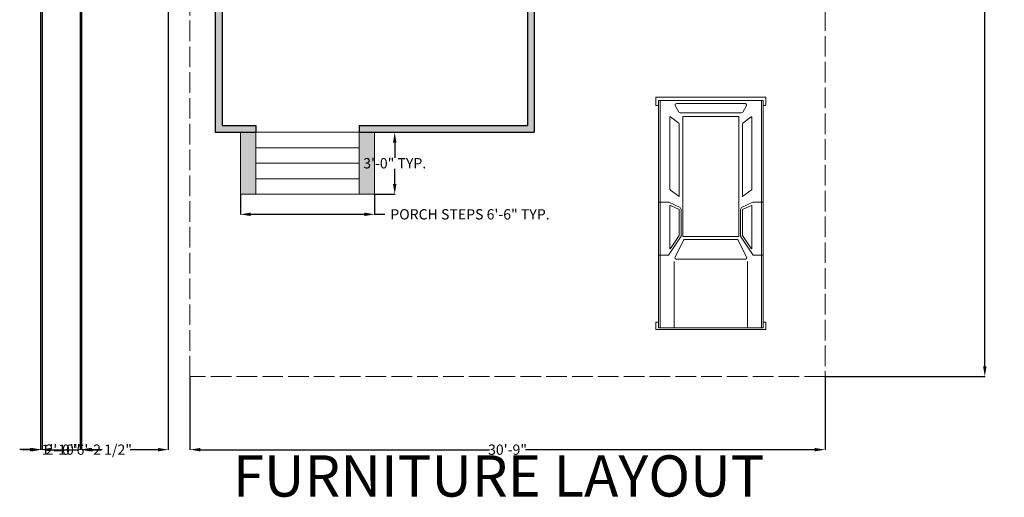
# Model space of a CAD drawing. Units: inches. Extents: x 1966 to 4198, y 2607 to 3884.
# Tile 4 of 8: x 2877 to 3450, y 3133 to 3411. Entities that reach past the tile are written whole.
import ezdxf

# ---------------------------------------------------------------- set-up
doc = ezdxf.new("R2010")
doc.units = ezdxf.units.IN
doc.header["$MEASUREMENT"] = 0
doc.linetypes.add('ACAD_ISO02W100', pattern=[15, 12, -3])
for name, color, linetype, lineweight in [('A-ANNO-TEXT', 4, 'Continuous', 25), ('A-FLOR', 7, 'Continuous', 25), ('A-FLOR-PATT', 9, 'Continuous', 13), ('A-FLOR-STRS', 7, 'Continuous', 18), ('A-WALL-PATT', 252, 'Continuous', 13), ('C-PRKG', 10, 'ACAD_ISO02W100', 18), ('C-PRKG-VEHI', 163, 'Continuous', 18), ('dimension', 90, 'Continuous', 18)]:
    doc.layers.add(name, color=color, linetype=linetype, lineweight=lineweight)
doc.styles.get("Standard").update_dxf_attribs({"font": 'arial.ttf'})
doc.dimstyles.get("Standard").update_dxf_attribs({"dimtxt": 6, "dimasz": 6, "dimexe": 0.18, "dimexo": 0.0625, "dimgap": 0.09, "dimtad": 0, "dimtih": 1, "dimtoh": 1, "dimdec": 1, "dimzin": 0, "dimdsep": 46, "dimlunit": 3, "dimtxsty": 'Standard', "dimcen": 0.09, "dimadec": 0, "dimazin": 0, "dimtfac": 1, "dimtdec": 1, "dimtofl": 0, "dimtmove": 0, "dimatfit": 3, "dimfxl": 1, "dimtolj": 1, "dimtzin": 0, "dimarcsym": 0})

# ---------------------------------------------------------------- blocks, each defined once
blk = doc.blocks.new('*U12')
for p, q in [((1.28, 38.87), (175.66, 38.87)), ((1.28, 28.15), (52.13, 28.15)), ((1.28, -28.15), (52.13, -28.15)), ((1.28, -38.87), (175.66, -38.87))]:
    blk.add_line(p, q)
for points in [[(5.57, 40.01), (5.57, 42.18), (0, 42.18), (0, -42.18), (5.57, -42.18), (5.57, -40.01), (1.28, -40.01), (1.28, 40.01)], [(1.28, 40.01), (175.66, 40.01), (175.66, -40.01), (1.28, -40.01)], [(171.74, 40.01), (175.66, 40.01), (175.66, -40.01), (171.74, -40.01), (171.74, -42.18), (178.14, -42.18), (178.14, 42.18), (171.74, 42.18)], [(71.47, 21.48), (163.42, 21.48), (163.42, -21.48), (71.47, -21.48)]]:
    blk.add_lwpolyline(points, close=True)
for points in [[(57.15, 40.01), (57.15, 32.39), (71.72, 22.83, 0.086577), (72.56, 22.68), (91.59, 22.68, 0.227875), (93.54, 23.62), (97.72, 32.11), (97.72, 40.01)], [(57.15, -40.01), (57.15, -32.39), (71.72, -22.83, -0.086577), (72.56, -22.68), (91.59, -22.68, -0.227875), (93.54, -23.62), (97.72, -32.11), (97.72, -40.01)]]:
    blk.add_lwpolyline(points, format="xyb")
for points in [[(62.08, 30.95), (72.14, 24.35, 0.146139), (72.69, 24.18), (91.42, 24.18, 0.29766), (92.33, 24.78), (95.09, 31.05, 0.541236), (94.86, 31.41), (62.21, 31.41, 0.744989)], [(102.19, 24.58), (106.97, 31, -0.236929), (107.78, 31.41), (162.91, 31.41, -0.621576), (163.11, 31), (158.19, 24.58, -0.233368), (157.39, 24.18), (102.39, 24.18, -0.616908)], [(55.49, 27.42), (68.59, 20.89, -0.284287), (69.14, 19.99), (69.14, -19.99, -0.284287), (68.59, -20.89), (55.49, -27.42, -0.557284), (54.05, -26.53), (54.05, 26.53, -0.557284)], [(171.88, 27.31), (166.83, 24.47, 0.271143), (166.32, 23.6), (166.32, -23.6, 0.271143), (166.83, -24.47), (171.88, -27.31, 0.573387), (173.37, -26.44), (173.37, 26.44, 0.573387)], [(62.08, -30.95), (72.14, -24.35, -0.146139), (72.69, -24.18), (91.42, -24.18, -0.29766), (92.33, -24.78), (95.09, -31.05, -0.541236), (94.86, -31.41), (62.21, -31.41, -0.744989)], [(102.19, -24.58), (106.97, -31, 0.236929), (107.78, -31.41), (162.91, -31.41, 0.621576), (163.11, -31), (158.19, -24.58, 0.233368), (157.39, -24.18), (102.39, -24.18, 0.616908)]]:
    blk.add_lwpolyline(points, format="xyb", close=True)
blk = doc.blocks.new('PORCH-ENTRY-STEPS')
for p, q in [((0, 36), (0, 0)), ((9, 36), (9, 0)), ((9, 36), (69, 36)), ((69, 0), (69, 36)), ((78, 0), (78, 36)), ((9, 27), (69, 27)), ((9, 18), (69, 18)), ((9, 9), (69, 9)), ((9, 0), (0, 0)), ((9, 0), (69, 0)), ((69, 0), (78, 0))]:
    blk.add_line(p, q)
blk = doc.blocks.new('PORCH-PARAPET-PLAN')
for p, q in [((0, 86), (0, 0)), ((4, 86), (4, 4)), ((181.42, 86), (181.42, 4)), ((185.42, 86), (185.42, 0)), ((0, 0), (23.64, 0)), ((4, 4), (23.64, 4)), ((23.64, 4), (23.64, 0)), ((83.64, 4), (83.64, 0)), ((83.64, 4), (181.42, 4)), ((83.64, 0), (185.42, 0))]:
    blk.add_line(p, q)
blk = doc.blocks.new('*D57')
at = {"layer": 'Defpoints', "color": 0, "transparency": 16777216}
for p in [(3005.67, 3309.5), (3083.67, 3309.5), (3083.67, 3297.8)]:
    blk.add_point(p, dxfattribs=at)
at = {"layer": 'dimension', "color": 0, "lineweight": -2, "transparency": 16777216}
for p, q in [((3005.67, 3309.44), (3005.67, 3297.62)), ((3083.67, 3309.44), (3083.67, 3297.62)), ((3011.67, 3297.8), (3077.67, 3297.8)), ((3083.67, 3297.8), (3089.67, 3297.8))]:
    blk.add_line(p, q, dxfattribs=at)
at = {"layer": 'dimension', "color": 0, "transparency": 16777216}
for points in [[(3011.67, 3298.8), (3011.67, 3296.8), (3005.67, 3297.8)], [(3077.67, 3298.8), (3077.67, 3296.8), (3083.67, 3297.8)]]:
    blk.add_solid(points, dxfattribs=at)
at = {"layer": 'dimension', "color": 0, "transparency": 16777216, "insert": (3139.1, 3297.8), "char_height": 6, "attachment_point": 5}
blk.add_mtext('\\A1;PORCH STEPS 6\'-6" TYP.', dxfattribs=at)
blk = doc.blocks.new('*D58')
at = {"layer": 'Defpoints', "color": 0, "transparency": 16777216}
for p in [(3083.67, 3345.5), (3095.37, 3345.5), (3083.67, 3309.5)]:
    blk.add_point(p, dxfattribs=at)
at = {"layer": 'dimension', "color": 0, "lineweight": -2, "transparency": 16777216}
for p, q in [((3083.73, 3345.5), (3095.55, 3345.5)), ((3095.37, 3339.5), (3095.37, 3330.66)), ((3095.37, 3315.5), (3095.37, 3324.35)), ((3083.73, 3309.5), (3095.55, 3309.5))]:
    blk.add_line(p, q, dxfattribs=at)
at = {"layer": 'dimension', "color": 0, "transparency": 16777216}
for points in [[(3094.37, 3339.5), (3096.37, 3339.5), (3095.37, 3345.5)], [(3094.37, 3315.5), (3096.37, 3315.5), (3095.37, 3309.5)]]:
    blk.add_solid(points, dxfattribs=at)
at = {"layer": 'dimension', "color": 0, "transparency": 16777216, "insert": (3095.37, 3327.5), "char_height": 6, "attachment_point": 5}
blk.add_mtext('\\A1;3\'-0" TYP.', dxfattribs=at)
blk = doc.blocks.new('*D88')
at = {"layer": 'Defpoints', "color": 0, "transparency": 16777216}
for p in [(3058.44, 3836.5), (3345.44, 3203.44), (3438.28, 3203.44)]:
    blk.add_point(p, dxfattribs=at)
at = {"layer": 'dimension', "color": 0, "lineweight": -2, "transparency": 16777216}
for p, q in [((3058.5, 3836.5), (3438.46, 3836.5)), ((3438.28, 3830.5), (3438.28, 3523.13)), ((3438.28, 3209.44), (3438.28, 3516.82)), ((3345.5, 3203.44), (3438.46, 3203.44))]:
    blk.add_line(p, q, dxfattribs=at)
at = {"layer": 'dimension', "color": 0, "transparency": 16777216}
for points in [[(3437.28, 3830.5), (3439.28, 3830.5), (3438.28, 3836.5)], [(3437.28, 3209.44), (3439.28, 3209.44), (3438.28, 3203.44)]]:
    blk.add_solid(points, dxfattribs=at)
at = {"layer": 'dimension', "color": 0, "transparency": 16777216, "insert": (3438.28, 3519.97), "char_height": 6, "attachment_point": 5}
blk.add_mtext('\\A1;52\'-9"', dxfattribs=at)
blk = doc.blocks.new('*D89')
at = {"layer": 'Defpoints', "color": 0, "transparency": 16777216}
for p in [(2976.4, 3203.44), (3345.44, 3203.44), (3345.44, 3160.93)]:
    blk.add_point(p, dxfattribs=at)
at = {"layer": 'dimension', "color": 0, "lineweight": -2, "transparency": 16777216}
for p, q in [((2976.4, 3203.38), (2976.4, 3160.75)), ((3345.44, 3203.38), (3345.44, 3160.75)), ((2982.4, 3160.93), (3150.53, 3160.93)), ((3339.44, 3160.93), (3171.31, 3160.93))]:
    blk.add_line(p, q, dxfattribs=at)
at = {"layer": 'dimension', "color": 0, "transparency": 16777216}
for points in [[(2982.4, 3161.93), (2982.4, 3159.93), (2976.4, 3160.93)], [(3339.44, 3161.93), (3339.44, 3159.93), (3345.44, 3160.93)]]:
    blk.add_solid(points, dxfattribs=at)
at = {"layer": 'dimension', "color": 0, "transparency": 16777216, "insert": (3160.92, 3160.93), "char_height": 6, "attachment_point": 5}
blk.add_mtext('\\A1;30\'-9"', dxfattribs=at)
blk = doc.blocks.new('*D90')
at = {"layer": 'Defpoints', "color": 0, "transparency": 16777216}
for p in [(2889.440566, 3668.990639), (2913.440566, 3668.990639), (2913.440566, 3160.931053)]:
    blk.add_point(p, dxfattribs=at)
at = {"layer": 'dimension', "color": 0, "lineweight": -2, "transparency": 16777216}
for p, q in [((2889.440566, 3668.928139), (2889.440566, 3160.751053)), ((2913.440566, 3668.928139), (2913.440566, 3160.751053)), ((2883.440566, 3160.931053), (2877.440566, 3160.931053)), ((2919.440566, 3160.931053), (2925.440566, 3160.931053))]:
    blk.add_line(p, q, dxfattribs=at)
at = {"layer": 'dimension', "color": 0, "transparency": 16777216}
for points in [[(2883.440566, 3161.931053), (2883.440566, 3159.931053), (2889.440566, 3160.931053)], [(2919.440566, 3161.931053), (2919.440566, 3159.931053), (2913.440566, 3160.931053)]]:
    blk.add_solid(points, dxfattribs=at)
at = {"layer": 'dimension', "color": 0, "transparency": 16777216, "insert": (2901.440566, 3160.931053), "char_height": 6, "attachment_point": 5}
blk.add_mtext('\\A1;2\'-0"', dxfattribs=at)
blk = doc.blocks.new('*D92')
at = {"layer": 'Defpoints', "color": 0, "transparency": 16777216}
for p in [(2889.44, 3623.5), (2963.74, 3623.5), (2963.74, 3160.93)]:
    blk.add_point(p, dxfattribs=at)
at = {"layer": 'dimension', "color": 0, "lineweight": -2, "transparency": 16777216}
for p, q in [((2889.44, 3623.44), (2889.44, 3160.75)), ((2963.74, 3623.44), (2963.74, 3160.75)), ((2895.44, 3160.93), (2911.52, 3160.93)), ((2957.74, 3160.93), (2941.66, 3160.93))]:
    blk.add_line(p, q, dxfattribs=at)
at = {"layer": 'dimension', "color": 0, "transparency": 16777216}
for points in [[(2895.44, 3161.93), (2895.44, 3159.93), (2889.44, 3160.93)], [(2957.74, 3161.93), (2957.74, 3159.93), (2963.74, 3160.93)]]:
    blk.add_solid(points, dxfattribs=at)
at = {"layer": 'dimension', "color": 0, "transparency": 16777216, "insert": (2926.59, 3160.93), "char_height": 6, "attachment_point": 5}
blk.add_mtext('\\A1;6\'-2 1/2"', dxfattribs=at)
blk = doc.blocks.new('*D97')
at = {"layer": 'Defpoints', "color": 0, "transparency": 16777216}
for p in [(2890.43, 3707.11), (2912.55, 3707.11), (2912.55, 3160.93)]:
    blk.add_point(p, dxfattribs=at)
at = {"layer": 'dimension', "color": 0, "lineweight": -2, "transparency": 16777216}
for p, q in [((2890.43, 3707.05), (2890.43, 3160.75)), ((2912.55, 3707.05), (2912.55, 3160.75)), ((2884.43, 3160.93), (2878.43, 3160.93)), ((2918.55, 3160.93), (2924.55, 3160.93))]:
    blk.add_line(p, q, dxfattribs=at)
at = {"layer": 'dimension', "color": 0, "transparency": 16777216}
for points in [[(2884.43, 3161.93), (2884.43, 3159.93), (2890.43, 3160.93)], [(2918.55, 3161.93), (2918.55, 3159.93), (2912.55, 3160.93)]]:
    blk.add_solid(points, dxfattribs=at)
at = {"layer": 'dimension', "color": 0, "transparency": 16777216, "insert": (2901.49, 3160.93), "char_height": 6, "attachment_point": 5}
blk.add_mtext('\\A1;1\'-10"', dxfattribs=at)

msp = doc.modelspace()

# ---------------------------------------------------------------- hatches: boundary and pattern name
at = {"layer": 'A-FLOR-PATT'}
h = msp.add_hatch(color=256, dxfattribs=at)
h.dxf.hatch_style = 1
h.paths.add_polyline_path([(3014.67, 3345.5), (3005.67, 3345.5), (3005.67, 3309.5), (3014.67, 3309.5)])
h.paths.add_polyline_path([(3083.67, 3345.5), (3074.67, 3345.5), (3074.67, 3309.5), (3083.67, 3309.5)])
at = {"layer": 'A-WALL-PATT'}
h = msp.add_hatch(color=256, dxfattribs=at)
h.dxf.hatch_style = 1
h.paths.add_polyline_path([(3010.44, 3599.5), (2889.44, 3599.5), (2889.44, 3698.62), (2880.44, 3698.62), (2880.44, 3590.5), (2880.44, 3539.5), (2889.44, 3539.5), (2889.44, 3590.5), (3010.44, 3590.5)])
h.paths.add_polyline_path([(2889.44, 3491.5), (2880.44, 3491.5), (2880.44, 3431.5), (2924.93, 3431.5), (2924.93, 3440.5), (2889.44, 3440.5)])
h.paths.add_polyline_path([(3008.43, 3440.5), (2972.93, 3440.5), (2972.93, 3431.5), (3008.43, 3431.5)])
h.paths.add_polyline_path([(2995.02, 3431.5), (2991.02, 3431.5), (2991.02, 3345.5), (3014.67, 3345.5), (3014.67, 3349.5), (2995.02, 3349.5)])
h.paths.add_polyline_path([(3232.44, 3440.5), (3176.44, 3440.5), (3176.44, 3587.5), (3183.92, 3587.5), (3183.92, 3591.41), (3183.92, 3596.5), (3167.44, 3596.5), (3167.44, 3440.5), (3092.44, 3440.5), (3092.44, 3590.5), (3083.44, 3590.5), (3083.44, 3440.5), (3056.43, 3440.5), (3056.43, 3438.68), (3056.43, 3431.5), (3092.44, 3431.5), (3232.44, 3431.5)])
h.paths.add_polyline_path([(3176.44, 3431.5), (3172.44, 3431.5), (3172.44, 3349.5), (3074.67, 3349.5), (3074.67, 3345.5), (3176.44, 3345.5)])
h.paths.add_polyline_path([(3345.44, 3490), (3336.44, 3490), (3336.44, 3440.5), (3280.44, 3440.5), (3280.44, 3431.5), (3345.44, 3431.5)])
h.paths.add_polyline_path([(3345.44, 3599.5), (3345.44, 3602.5), (3336.44, 3602.5), (3336.44, 3596.5), (3296.55, 3596.5), (3296.55, 3587.5), (3336.44, 3587.5), (3336.44, 3538), (3345.44, 3538)])
h.paths.add_polyline_path([(3264.44, 3632.5), (3336.44, 3632.5), (3336.44, 3626.5), (3345.44, 3626.5), (3345.44, 3692.5), (3336.44, 3692.5), (3336.44, 3641.5), (3219.92, 3641.5), (3219.92, 3632.5), (3258.44, 3632.5), (3258.44, 3596.5), (3219.95, 3596.5), (3219.95, 3591.41, -0.010779), (3219.92, 3589.86), (3219.92, 3587.5), (3268.55, 3587.5), (3268.55, 3591.7), (3268.55, 3596.5), (3264.44, 3596.5)])
h.paths.add_polyline_path([(3175.44, 3791.5), (3231.94, 3791.5), (3231.94, 3800.5), (3175.44, 3800.5), (3154.44, 3800.5), (3154.44, 3791.5), (3166.44, 3791.5), (3166.44, 3719.5), (3118.44, 3719.5), (3112.44, 3719.5), (3058.44, 3719.5), (3058.44, 3710.5), (3166.44, 3710.5), (3166.44, 3632.5), (3183.92, 3632.5), (3183.92, 3637.87), (3183.92, 3641.5), (3175.44, 3641.5)])
h.paths.add_polyline_path([(3345.44, 3800.5), (3279.94, 3800.5), (3279.94, 3791.5), (3336.44, 3791.5), (3336.44, 3740.5), (3345.44, 3740.5)])
h.paths.add_polyline_path([(3130.44, 3800.5), (3100.44, 3800.5), (3100.44, 3791.5), (3112.44, 3791.5), (3112.44, 3755.5), (3112.44, 3751.71), (3112.44, 3747.5), (3118.44, 3747.5), (3118.44, 3791.5), (3130.44, 3791.5)], flags=17)
h.paths.add_polyline_path([(3076.44, 3800.5), (3058.44, 3800.5), (3058.44, 3796.92), (3058.44, 3791.5), (3058.44, 3749.5), (3084.38, 3749.5), (3084.38, 3751.71, -0.016709), (3084.44, 3753.59), (3084.44, 3755.5), (3064.44, 3755.5), (3064.44, 3791.5), (3076.44, 3791.5)], flags=17)
h.paths.add_polyline_path([(3022.36, 3796.92, -0.017138), (3022.44, 3799.39), (3022.44, 3800.5), (3010.44, 3800.5), (2969.44, 3800.5), (2969.44, 3791.5), (3001.44, 3791.5), (3001.44, 3632.5), (3010.44, 3632.5), (3010.44, 3791.5), (3022.36, 3791.5)])
h.paths.add_polyline_path([(2921.44, 3800.5), (2880.44, 3800.5), (2880.44, 3746.62), (2889.44, 3746.62), (2889.44, 3791.5), (2921.44, 3791.5)])

# ---------------------------------------------------------------- linework, layer by layer
at = {"layer": 'C-PRKG'}
for p, q in [((2976.4, 3203.44), (2976.4, 3431.5)), ((3345.44, 3431.5), (3345.44, 3203.44)), ((3345.44, 3203.44), (2976.4, 3203.44))]:
    msp.add_line(p, q, dxfattribs=at)

# ---------------------------------------------------------------- block references
at = {"layer": 'A-FLOR'}
msp.add_blockref('PORCH-PARAPET-PLAN', (2991.02, 3345.5), dxfattribs=at)
at = {"layer": 'A-FLOR-STRS'}
msp.add_blockref('PORCH-ENTRY-STEPS', (3005.67, 3309.5), dxfattribs=at)
at = {"layer": 'C-PRKG-VEHI', "xscale": 0.7580236284792754, "yscale": 0.7580236284792754, "zscale": 0.7580236284792754, "rotation": 90}
msp.add_blockref('*U12', (3279.07, 3230.82), dxfattribs=at)

# ---------------------------------------------------------------- texts
at = {"layer": 'A-ANNO-TEXT', "insert": (3155.76, 3157.64), "char_height": 24, "attachment_point": 2}
msp.add_mtext_dynamic_manual_height_columns('FURNITURE LAYOUT', width=388.1177, gutter_width=1, heights=[0], dxfattribs=at)

# ---------------------------------------------------------------- dimensions: what is measured, and where the dimension line sits
at = {"layer": 'dimension'}
dim = msp.add_linear_dim(base=(3438.28, 3203.44), p1=(3058.44, 3836.5), p2=(3345.44, 3203.44), angle=90, dimstyle='Standard', override={"dimdec": 1, "dimlfac": 1, "dimrnd": 0, "dimzin": 1, "dimdsep": 46, "dimlunit": 4, "dimfrac": 2}, dxfattribs=at)
dim.commit()
dim.dimension.update_dxf_attribs({"geometry": '*D88', "text_midpoint": (3438.28, 3519.97)})
for base, p1, p2, picture, middle in [((2912.55, 3160.93), (2890.43, 3707.11), (2912.55, 3707.11), '*D97', (2901.49, 3160.93)), ((2913.44, 3160.93), (2889.44, 3668.99), (2913.44, 3668.99), '*D90', (2901.44, 3160.93)), ((2963.74, 3160.93), (2889.44, 3623.5), (2963.74, 3623.5), '*D92', (2926.59, 3160.93)), ((3345.44, 3160.93), (2976.4, 3203.44), (3345.44, 3203.44), '*D89', (3160.92, 3160.93))]:
    dim = msp.add_linear_dim(base=base, p1=p1, p2=p2, dimstyle='Standard', override={"dimdec": 1, "dimlfac": 1, "dimrnd": 0, "dimzin": 1, "dimdsep": 46, "dimlunit": 4, "dimfrac": 2}, dxfattribs=at)
    dim.commit()
    dim.dimension.update_dxf_attribs({"geometry": picture, "text_midpoint": middle})
dim = msp.add_linear_dim(base=(3095.37, 3345.5), p1=(3083.67, 3309.5), p2=(3083.67, 3345.5), angle=90, text='<> TYP.', dimstyle='Standard', override={"dimdec": 1, "dimlfac": 1, "dimrnd": 0, "dimzin": 1, "dimdsep": 46, "dimlunit": 4, "dimfrac": 2}, dxfattribs=at)
dim.commit()
dim.dimension.update_dxf_attribs({"geometry": '*D58', "text_midpoint": (3095.37, 3327.5)})
dim = msp.add_linear_dim(base=(3083.67, 3297.8), p1=(3005.67, 3309.5), p2=(3083.67, 3309.5), text='PORCH STEPS <> TYP.', dimstyle='Standard', override={"dimdec": 1, "dimlfac": 1, "dimrnd": 0, "dimzin": 1, "dimdsep": 46, "dimlunit": 4, "dimfrac": 2}, dxfattribs=at)
dim.commit()
dim.dimension.update_dxf_attribs({"geometry": '*D57', "text_midpoint": (3139.1, 3297.8)})

doc.saveas('drawing.dxf')
